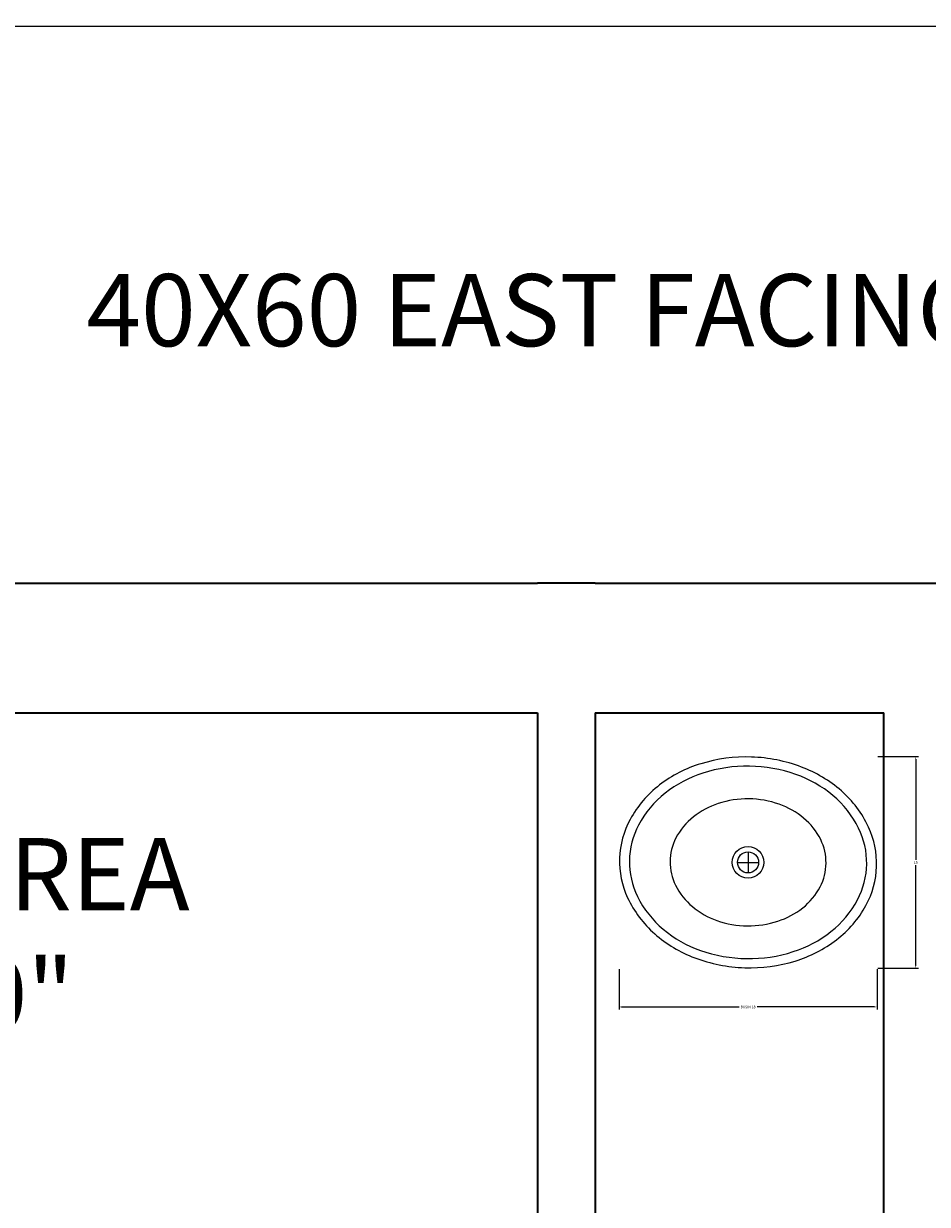
# Model space of a CAD drawing. Units: inches. Extents: x -86 to 2463, y -1058 to 68.
# Tile 16 of 17: x 85 to 148, y -14 to 68. Entities that reach past the tile are written whole.
import ezdxf

# ---------------------------------------------------------------- set-up
doc = ezdxf.new("R2010")
doc.units = ezdxf.units.IN
doc.header["$MEASUREMENT"] = 0
for name, color, linetype, lineweight in [('A-ANNO-DIMS', 2, 'Continuous', 18), ('A-ANNO-TITL', 7, 'Continuous', 25), ('A-AREA-IDEN', 7, 'Continuous', 18), ('A-FLOR-FIXT', 9, 'Continuous', 18), ('A-WALL', 7, 'Continuous', 35)]:
    doc.layers.add(name, color=color, linetype=linetype, lineweight=lineweight)
doc.styles.get("Standard").update_dxf_attribs({"font": 'arial.ttf'})
doc.dimstyles.get("Standard").update_dxf_attribs({"dimtxt": 0.18, "dimasz": 0.18, "dimexe": 0.18, "dimexo": 0.0625, "dimgap": 0.09, "dimtad": 0, "dimtih": 1, "dimtoh": 1, "dimdec": 4, "dimzin": 0, "dimdsep": 46, "dimtxsty": 'Standard', "dimcen": 0.09, "dimadec": 0, "dimazin": 0, "dimtfac": 1, "dimtdec": 4, "dimtofl": 0, "dimtmove": 0, "dimatfit": 3, "dimfxl": 1, "dimtolj": 1, "dimtzin": 0, "dimarcsym": 0})

# ---------------------------------------------------------------- blocks, each defined once
blk = doc.blocks.new('Sink - Oval top')
for p, q in [((-1, 0), (1, 0)), ((0, 1), (0, -1))]:
    blk.add_line(p, q)
for points in [[(-12.23, 0.39, 0.117634), (-11.46, -3.36, 0.104469), (-8.88, -6.8, 0.090016), (-5.08, -9.07, 0.08192), (-0.32, -10.02, 0.08192), (4.49, -9.38, 0.090016), (8.42, -7.36, 0.104469), (11.22, -4.09, 0.117634), (12.23, -0.39, 0.117634), (11.46, 3.36, 0.104469), (8.88, 6.8, 0.090016), (5.08, 9.07, 0.08192), (0.32, 10.02, 0.08192), (-4.49, 9.38, 0.090016), (-8.42, 7.36, 0.104469), (-11.22, 4.09, 0.117634)], [(-11.29, 0.16, 0.118622), (-10.52, -3.25, 0.104678), (-8.07, -6.36, 0.089562), (-4.54, -8.37, 0.081185), (-0.13, -9.15, 0.081185), (4.3, -8.49, 0.089562), (7.89, -6.58, 0.104678), (10.42, -3.55, 0.118622), (11.29, -0.16, 0.118622), (10.52, 3.25, 0.104678), (8.07, 6.36, 0.089562), (4.54, 8.37, 0.081185), (0.13, 9.15, 0.081185), (-4.3, 8.49, 0.089562), (-7.89, 6.58, 0.104678), (-10.42, 3.55, 0.118622)], [(-7.42, 0.08, 0.118283), (-6.91, -2.17, 0.104607), (-5.29, -4.21, 0.089718), (-2.97, -5.53, 0.081436), (-0.07, -6.04, 0.081436), (2.84, -5.59, 0.089718), (5.2, -4.33, 0.104607), (6.86, -2.32, 0.118283), (7.42, -0.08, 0.118283), (6.91, 2.17, 0.104607), (5.29, 4.21, 0.089718), (2.97, 5.53, 0.081436), (0.07, 6.04, 0.081436), (-2.84, 5.59, 0.089718), (-5.2, 4.33, 0.104607), (-6.86, 2.32, 0.118283)]]:
    blk.add_lwpolyline(points, format="xyb", close=True)
for radius in [1.5, 1]:
    blk.add_circle((0, 0), radius)
blk = doc.blocks.new('*D18')
at = {"layer": 'A-ANNO-DIMS', "color": 0, "lineweight": -2, "transparency": 16777216}
for p, q in [((126.407, 2.127), (126.407, -0.675)), ((144.303, 2.127), (144.303, -0.675)), ((126.587, -0.495), (134.728, -0.495)), ((144.123, -0.495), (135.982, -0.495))]:
    blk.add_line(p, q, dxfattribs=at)
at = {"layer": 'A-ANNO-DIMS', "color": 0, "transparency": 16777216}
for points in [[(126.587, -0.465), (126.587, -0.525), (126.407, -0.495)], [(144.123, -0.465), (144.123, -0.525), (144.303, -0.495)]]:
    blk.add_solid(points, dxfattribs=at)
at = {"layer": 'Defpoints', "color": 0, "transparency": 16777216}
for p in [(126.407, 2.189), (144.303, 2.189), (144.303, -0.495)]:
    blk.add_point(p, dxfattribs=at)
at = {"layer": 'A-ANNO-DIMS', "color": 0, "transparency": 16777216, "insert": (135.355, -0.495), "char_height": 0.18, "attachment_point": 5}
blk.add_mtext('\\A1;BASIN 18', dxfattribs=at)
blk = doc.blocks.new('*D19')
at = {"layer": 'A-ANNO-DIMS', "color": 0, "lineweight": -2, "transparency": 16777216}
for p, q in [((144.365, 16.867), (147.167, 16.867)), ((146.987, 16.687), (146.987, 9.71)), ((146.987, 2.369), (146.987, 9.346)), ((144.365, 2.189), (147.167, 2.189))]:
    blk.add_line(p, q, dxfattribs=at)
at = {"layer": 'A-ANNO-DIMS', "color": 0, "transparency": 16777216}
for points in [[(146.957, 16.687), (147.017, 16.687), (146.987, 16.867)], [(146.957, 2.369), (147.017, 2.369), (146.987, 2.189)]]:
    blk.add_solid(points, dxfattribs=at)
at = {"layer": 'Defpoints', "color": 0, "transparency": 16777216}
for p in [(144.303, 16.867), (146.987, 16.867), (144.303, 2.189)]:
    blk.add_point(p, dxfattribs=at)
at = {"layer": 'A-ANNO-DIMS', "color": 0, "transparency": 16777216, "insert": (146.987, 9.528), "char_height": 0.18, "attachment_point": 5}
blk.add_mtext('\\A1;15', dxfattribs=at)
blk = doc.blocks.new('*D35')
at = {"layer": 'A-ANNO-DIMS', "color": 0, "lineweight": -2, "transparency": 16777216}
for p, q in [((15.761, 28.958), (15.761, 67.676)), ((15.941, 67.496), (200.989, 67.496)), ((386.581, 67.496), (201.532, 67.496)), ((386.761, 28.958), (386.761, 67.676))]:
    blk.add_line(p, q, dxfattribs=at)
at = {"layer": 'A-ANNO-DIMS', "color": 0, "transparency": 16777216}
for points in [[(15.941, 67.526), (15.941, 67.466), (15.761, 67.496)], [(386.581, 67.526), (386.581, 67.466), (386.761, 67.496)]]:
    blk.add_solid(points, dxfattribs=at)
at = {"layer": 'Defpoints', "color": 0, "transparency": 16777216}
for p in [(386.761, 67.496), (15.761, 28.896), (386.761, 28.896)]:
    blk.add_point(p, dxfattribs=at)
at = {"layer": 'A-ANNO-DIMS', "color": 0, "transparency": 16777216, "insert": (201.261, 67.496), "char_height": 0.18, "attachment_point": 5}
blk.add_mtext('\\A1;371', dxfattribs=at)

msp = doc.modelspace()

# ---------------------------------------------------------------- linework, layer by layer
at = {"layer": 'A-WALL'}
for p, q in [((24.761, 28.896), (120.761, 28.896)), ((124.761, 28.896), (120.761, 28.896)), ((124.761, 28.896), (386.761, 28.896)), ((24.761, 19.896), (120.761, 19.896)), ((120.761, 19.896), (120.761, -16.104)), ((124.761, 19.896), (124.761, -61.399)), ((124.761, 19.896), (144.761, 19.896)), ((144.761, -32.104), (144.761, 19.896))]:
    msp.add_line(p, q, dxfattribs=at)

# ---------------------------------------------------------------- block references
at = {"layer": 'A-FLOR-FIXT', "xscale": 0.7289195526103346, "yscale": 0.7289195526103346, "zscale": 0.7289195526103346}
msp.add_blockref('Sink - Oval top', (135.355, 9.528), dxfattribs=at)

# ---------------------------------------------------------------- texts
at = {"layer": 'A-ANNO-TITL', "insert": (89.471, 50.312), "char_height": 5, "attachment_point": 1}
msp.add_mtext_dynamic_manual_height_columns('40X60 EAST FACING APARTMENT HOUSE PLAN', width=543.41592, gutter_width=25, heights=[0], dxfattribs=at)
at = {"layer": 'A-AREA-IDEN', "insert": (59.281, 11.211), "char_height": 5, "attachment_point": 1}
msp.add_mtext_dynamic_manual_height_columns('WASH AREA\\P8\'0"X3\'0"', width=81.49318, gutter_width=25, heights=[0], dxfattribs=at)

# ---------------------------------------------------------------- dimensions: what is measured, and where the dimension line sits
at = {"layer": 'A-ANNO-DIMS'}
dim = msp.add_linear_dim(base=(386.761, 67.496), p1=(15.761, 28.896), p2=(386.761, 28.896), dimstyle='Standard', override={"dimdec": 0, "dimlfac": 1, "dimrnd": 0, "dimzin": 0, "dimdsep": 46, "dimlunit": 2}, dxfattribs=at)
dim.commit()
dim.dimension.update_dxf_attribs({"geometry": '*D35', "text_midpoint": (201.261, 67.496)})
dim = msp.add_linear_dim(base=(146.987, 16.867), p1=(144.303, 2.189), p2=(144.303, 16.867), angle=90, dimstyle='Standard', override={"dimdec": 0, "dimlfac": 1, "dimrnd": 0, "dimzin": 0, "dimdsep": 46, "dimlunit": 2}, dxfattribs=at)
dim.commit()
dim.dimension.update_dxf_attribs({"geometry": '*D19', "text_midpoint": (146.987, 9.528)})
dim = msp.add_linear_dim(base=(144.303, -0.495), p1=(126.407, 2.189), p2=(144.303, 2.189), text='BASIN <>', dimstyle='Standard', override={"dimdec": 0, "dimlfac": 1, "dimrnd": 0, "dimzin": 0, "dimdsep": 46, "dimlunit": 2}, dxfattribs=at)
dim.commit()
dim.dimension.update_dxf_attribs({"geometry": '*D18', "text_midpoint": (135.355, -0.495)})

doc.saveas('drawing.dxf')
